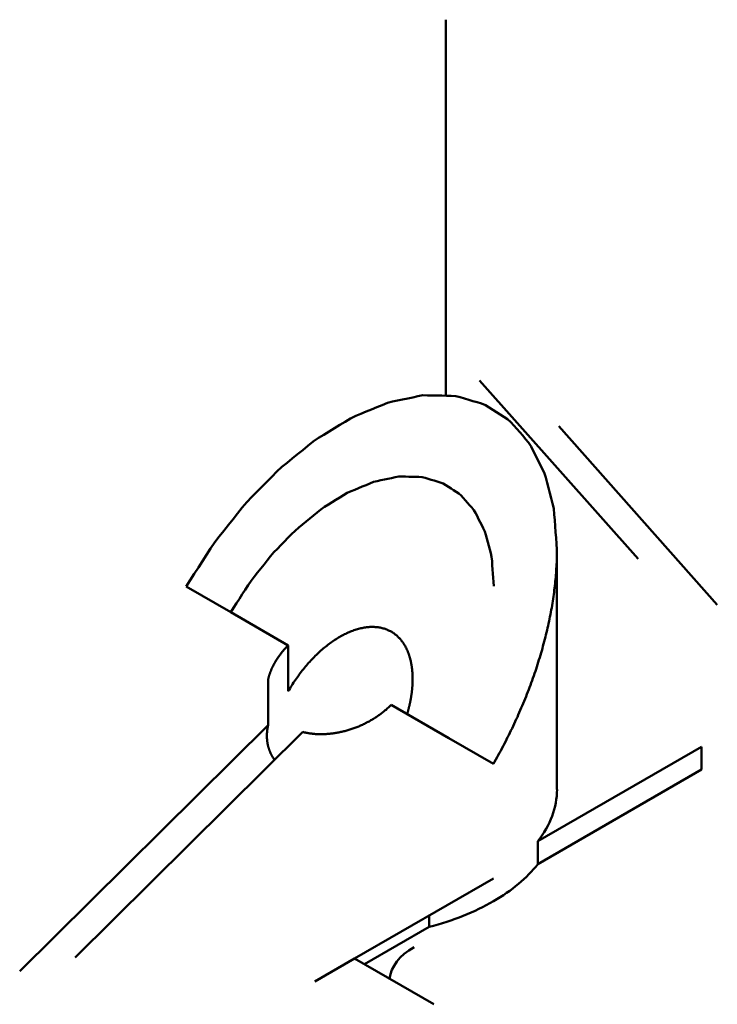
# Model space of a CAD drawing. Units: inches. Extents: x 181 to 9700, y 72 to 10161.
# Tile 2 of 2: x 5829 to 9700, y 4700 to 10161. Entities that reach past the tile are written whole.
import ezdxf

# ---------------------------------------------------------------- set-up
doc = ezdxf.new("R2010")
doc.units = ezdxf.units.IN
doc.header["$MEASUREMENT"] = 0
doc.layers.add('M-OUTL', color=7, linetype='Continuous', lineweight=50)

msp = doc.modelspace()

# ---------------------------------------------------------------- linework, layer by layer
at = {"layer": 'M-OUTL'}
for p, q in [((8193.3, 8080.4), (8193.3, 10161.2)), ((9260.1, 7170.3), (8380.2, 8160.9)), ((9700.1, 6916.3), (8820.2, 7906.9)), ((8810.3, 7221.8), (8810.3, 5890.8)), ((6999.9, 6875), (6752.5, 7017.9)), ((7318.9, 6690.9), (6999.9, 6875)), ((7318.9, 6436.9), (7318.9, 6690.9)), ((7207.6, 6249.2), (7207.6, 6503.2)), ((8209.8, 6176.5), (7890.8, 6360.7)), ((5828.6, 4884.3), (7207.6, 6249.2)), ((7399.5, 6210.5), (6136.6, 4960.5)), ((8457.2, 6033.7), (8209.8, 6176.5)), ((8703.5, 5604.3), (9612.1, 6128.9)), ((9612.1, 6001.9), (9612.1, 6128.9)), ((8703.5, 5477.3), (9612.1, 6001.9)), ((8703.5, 5477.3), (8703.5, 5604.3)), ((8457.2, 5398.7), (7687.3, 4954.2)), ((8101, 5129.5), (8101, 5193)), ((7742.3, 4922.4), (8101, 5129.5)), ((7467.4, 4827.2), (7687.3, 4954.2)), ((8127.3, 4700.2), (7687.3, 4954.2))]:
    msp.add_line(p, q, dxfattribs=at)
for points in [[(6752.5, 7017.9), (6775, 7053), (6797.6, 7088), (6820.2, 7123.1), (6842.8, 7158.1), (6865.4, 7193.2), (6887.9, 7228.2), (6910.9, 7262.8), (6936.4, 7294.9), (6961.8, 7326.9), (6987.3, 7358.9), (7012.7, 7391), (7038.2, 7423), (7063.6, 7455), (7089.7, 7485.9), (7117.3, 7514.1), (7144.9, 7542.2), (7172.5, 7570.3), (7200.1, 7598.4), (7227.8, 7626.5), (7255.4, 7654.6), (7283.6, 7680.7), (7312.5, 7704.1), (7341.5, 7727.5), (7370.5, 7750.9), (7399.5, 7774.3), (7428.5, 7797.6), (7457.5, 7821), (7486.8, 7841.3), (7516.3, 7859.4), (7545.8, 7877.4), (7575.4, 7895.4), (7604.9, 7913.4), (7634.5, 7931.4), (7664, 7949.4), (7693.3, 7963.2), (7722.6, 7975.4), (7751.9, 7987.5), (7781.1, 7999.6), (7810.4, 8011.7), (7839.7, 8023.8), (7868.9, 8036), (7897.2, 8042.8), (7925.4, 8048.6), (7953.5, 8054.5), (7981.7, 8060.4), (8009.8, 8066.3), (8038, 8072.2), (8066.2, 8078.1), (8092.4, 8077.6), (8118.7, 8077.1), (8144.9, 8076.6), (8171.2, 8076.1), (8197.4, 8075.6), (8223.7, 8075.1), (8249.6, 8073.7), (8273.2, 8066.8), (8296.8, 8059.9), (8320.4, 8053), (8344, 8046.1), (8367.6, 8039.2), (8391.2, 8032.4), (8413.9, 8023.7), (8434.2, 8010.6), (8454.5, 7997.6), (8474.8, 7984.5), (8495.1, 7971.4), (8515.4, 7958.3), (8535.7, 7945.3), (8554.4, 7929.7), (8570.8, 7910.8), (8587.2, 7891.9), (8603.6, 7873), (8620, 7854.1), (8636.4, 7835.2), (8652.9, 7816.3), (8666.8, 7794.4), (8678.9, 7770.2), (8690.9, 7746.1), (8703, 7721.9), (8715.1, 7697.7), (8727.1, 7673.5), (8739.2, 7649.3), (8747.9, 7621.9), (8755.3, 7593.1), (8762.7, 7564.3), (8770.1, 7535.5), (8777.5, 7506.8), (8784.8, 7478), (8792.2, 7449.2), (8795.4, 7417.2), (8797.9, 7384.6), (8800.4, 7352), (8802.9, 7319.5), (8805.3, 7286.9), (8807.8, 7254.3), (8810.3, 7221.8)], [(6999.9, 6875), (7016, 6899.9), (7032, 6924.8), (7048, 6949.7), (7064, 6974.5), (7080.1, 6999.4), (7096.1, 7024.3), (7112.4, 7048.9), (7130.5, 7071.6), (7148.5, 7094.3), (7166.6, 7117.1), (7184.6, 7139.8), (7202.7, 7162.5), (7220.8, 7185.3), (7239.3, 7207.2), (7258.9, 7227.1), (7278.5, 7247.1), (7298.1, 7267), (7317.6, 7287), (7337.2, 7306.9), (7356.8, 7326.9), (7376.8, 7345.4), (7397.4, 7362), (7418, 7378.6), (7438.5, 7395.2), (7459.1, 7411.8), (7479.7, 7428.4), (7500.3, 7445), (7521, 7459.4), (7542, 7472.2), (7563, 7485), (7583.9, 7497.8), (7604.9, 7510.5), (7625.9, 7523.3), (7646.8, 7536.1), (7667.7, 7545.9), (7688.4, 7554.5), (7709.2, 7563.1), (7730, 7571.7), (7750.7, 7580.3), (7771.5, 7588.9), (7792.3, 7597.5), (7812.3, 7602.3), (7832.3, 7606.5), (7852.3, 7610.7), (7872.3, 7614.9), (7892.3, 7619.1), (7912.3, 7623.3), (7932.2, 7627.4), (7950.9, 7627.1), (7969.5, 7626.7), (7988.1, 7626.4), (8006.8, 7626), (8025.4, 7625.7), (8044, 7625.3), (8062.4, 7624.3), (8079.1, 7619.4), (8095.9, 7614.5), (8112.7, 7609.6), (8129.4, 7604.7), (8146.2, 7599.9), (8162.9, 7595), (8179, 7588.8), (8193.4, 7579.5), (8207.8, 7570.3), (8222.2, 7561), (8236.6, 7551.7), (8251.1, 7542.4), (8265.5, 7533.2), (8278.7, 7522.1), (8290.3, 7508.7), (8302, 7495.3), (8313.6, 7481.9), (8325.3, 7468.5), (8336.9, 7455.1), (8348.6, 7441.7), (8358.5, 7426.1), (8367.1, 7408.9), (8375.6, 7391.8), (8384.2, 7374.6), (8392.8, 7357.5), (8401.3, 7340.3), (8409.9, 7323.2), (8416.1, 7303.7), (8421.3, 7283.2), (8426.5, 7262.8), (8431.8, 7242.4), (8437, 7222), (8442.3, 7201.5), (8447.5, 7181.1), (8449.8, 7158.4), (8451.5, 7135.3), (8453.3, 7112.2), (8455, 7089), (8456.8, 7065.9), (8458.6, 7042.8), (8460.3, 7019.7)], [(8810.3, 7221.8), (8810, 7210.2), (8809.8, 7198.7), (8809.5, 7187.1), (8809.2, 7175.6), (8808.9, 7164.1), (8808.6, 7152.5), (8808.3, 7140.9), (8807.5, 7129.1), (8806.6, 7117.3), (8805.8, 7105.5), (8805, 7093.6), (8804.1, 7081.8), (8803.3, 7070), (8802.3, 7058.1), (8801, 7046), (8799.6, 7034), (8798.2, 7021.9), (8796.8, 7009.8), (8795.4, 6997.7), (8794.1, 6985.7), (8792.5, 6973.5), (8790.5, 6961.2), (8788.6, 6949), (8786.7, 6936.7), (8784.8, 6924.4), (8782.8, 6912.1), (8780.9, 6899.8), (8778.7, 6887.5), (8776.2, 6875), (8773.8, 6862.6), (8771.3, 6850.1), (8768.8, 6837.7), (8766.4, 6825.2), (8763.9, 6812.8), (8761.1, 6800.2), (8758.1, 6787.7), (8755.1, 6775.1), (8752.1, 6762.5), (8749.1, 6749.9), (8746.1, 6737.4), (8743.1, 6724.8), (8739.6, 6712.1), (8736.1, 6699.5), (8732.6, 6686.8), (8729.1, 6674.1), (8725.6, 6661.4), (8722.1, 6648.8), (8718.5, 6636.1), (8714.5, 6623.4), (8710.5, 6610.7), (8706.5, 6598), (8702.4, 6585.2), (8698.4, 6572.5), (8694.4, 6559.8), (8690.3, 6547.1), (8685.8, 6534.4), (8681.2, 6521.6), (8676.7, 6508.9), (8672.2, 6496.2), (8667.7, 6483.4), (8663.1, 6470.7), (8658.5, 6458), (8653.5, 6445.3), (8648.4, 6432.6), (8643.4, 6419.9), (8638.4, 6407.2), (8633.4, 6394.5), (8628.4, 6381.8), (8623.2, 6369.1), (8617.7, 6356.5), (8612.2, 6343.9), (8606.8, 6331.2), (8601.3, 6318.6), (8595.8, 6306), (8590.3, 6293.3), (8584.6, 6280.8), (8578.7, 6268.2), (8572.7, 6255.7), (8566.8, 6243.2), (8560.9, 6230.7), (8554.9, 6218.2), (8549, 6205.6), (8542.8, 6193.2), (8536.4, 6180.9), (8530, 6168.5), (8523.7, 6156.1), (8517.3, 6143.7), (8511, 6131.4), (8504.6, 6119), (8497.9, 6106.8), (8491.1, 6094.6), (8484.3, 6082.4), (8477.6, 6070.2), (8470.8, 6058), (8464, 6045.9), (8457.2, 6033.7)], [(7318.9, 6436.9), (7323.8, 6444.8), (7328.8, 6452.8), (7333.7, 6460.7), (7338.6, 6468.6), (7343.5, 6476.6), (7348.5, 6484.5), (7353.5, 6492.4), (7358.9, 6499.9), (7364.3, 6507.5), (7369.7, 6515), (7375.1, 6522.5), (7380.4, 6530.1), (7385.8, 6537.6), (7391.3, 6545), (7397.1, 6552), (7402.9, 6559.1), (7408.7, 6566.1), (7414.5, 6573.1), (7420.3, 6580.2), (7426.1, 6587.2), (7432, 6594), (7438.1, 6600.4), (7444.2, 6606.9), (7450.3, 6613.3), (7456.4, 6619.8), (7462.6, 6626.2), (7468.7, 6632.7), (7474.9, 6638.8), (7481.3, 6644.5), (7487.6, 6650.3), (7494, 6656.1), (7500.3, 6661.9), (7506.7, 6667.7), (7513, 6673.5), (7519.5, 6678.7), (7526, 6683.7), (7532.6, 6688.8), (7539.1, 6693.8), (7545.6, 6698.9), (7552.1, 6703.9), (7558.6, 6709), (7565.2, 6713.3), (7571.8, 6717.6), (7578.4, 6721.8), (7585, 6726), (7591.6, 6730.3), (7598.3, 6734.5), (7604.9, 6738.8), (7611.5, 6742.2), (7618.1, 6745.5), (7624.7, 6748.9), (7631.3, 6752.3), (7637.9, 6755.7), (7644.5, 6759.1), (7651.1, 6762.3), (7657.6, 6764.8), (7664.1, 6767.3), (7670.6, 6769.8), (7677.1, 6772.3), (7683.7, 6774.8), (7690.2, 6777.2), (7696.7, 6779.5), (7703, 6781), (7709.4, 6782.6), (7715.7, 6784.1), (7722.1, 6785.7), (7728.4, 6787.2), (7734.8, 6788.8), (7741, 6789.9), (7747.2, 6790.5), (7753.3, 6791.1), (7759.4, 6791.8), (7765.5, 6792.4), (7771.6, 6793), (7777.7, 6793.6), (7783.6, 6793.6), (7789.4, 6793.3), (7795.2, 6792.9), (7801, 6792.6), (7806.8, 6792.2), (7812.6, 6791.9), (7818.4, 6791.5), (7823.9, 6790.5), (7829.3, 6789.2), (7834.7, 6787.9), (7840, 6786.6), (7845.4, 6785.3), (7850.8, 6784), (7856.2, 6782.7), (7861.2, 6780.5), (7866.2, 6778.3), (7871.1, 6776.1), (7876, 6773.8), (7881, 6771.6), (7885.9, 6769.3), (7890.8, 6767.1)], [(7890.8, 6767.1), (7893.1, 6765.6), (7895.4, 6764.2), (7897.6, 6762.7), (7899.9, 6761.2), (7902.2, 6759.8), (7904.5, 6758.3), (7906.7, 6756.8), (7908.8, 6755.1), (7911, 6753.4), (7913.1, 6751.8), (7915.2, 6750.1), (7917.4, 6748.4), (7919.5, 6746.7), (7921.6, 6744.9), (7923.6, 6743), (7925.6, 6741.1), (7927.6, 6739.2), (7929.6, 6737.3), (7931.5, 6735.4), (7933.5, 6733.5), (7935.5, 6731.5), (7937.3, 6729.4), (7939.1, 6727.3), (7941, 6725.2), (7942.8, 6723.1), (7944.7, 6721), (7946.5, 6718.8), (7948.2, 6716.6), (7949.9, 6714.3), (7951.6, 6712), (7953.3, 6709.7), (7955, 6707.3), (7956.6, 6705), (7958.3, 6702.7), (7959.9, 6700.2), (7961.4, 6697.7), (7962.9, 6695.2), (7964.4, 6692.7), (7966, 6690.2), (7967.5, 6687.6), (7969, 6685.1), (7970.4, 6682.4), (7971.7, 6679.7), (7973.1, 6677), (7974.4, 6674.3), (7975.8, 6671.6), (7977.1, 6668.9), (7978.5, 6666.2), (7979.7, 6663.3), (7980.8, 6660.4), (7982, 6657.5), (7983.2, 6654.7), (7984.4, 6651.8), (7985.6, 6648.9), (7986.7, 6646), (7987.7, 6642.9), (7988.7, 6639.9), (7989.7, 6636.8), (7990.7, 6633.7), (7991.7, 6630.7), (7992.7, 6627.6), (7993.7, 6624.5), (7994.5, 6621.3), (7995.3, 6618.1), (7996.2, 6614.8), (7997, 6611.6), (7997.8, 6608.4), (7998.7, 6605.2), (7999.4, 6601.9), (8000, 6598.5), (8000.7, 6595.1), (8001.3, 6591.8), (8002, 6588.4), (8002.6, 6585), (8003.3, 6581.6), (8003.8, 6578.2), (8004.3, 6574.7), (8004.7, 6571.2), (8005.2, 6567.6), (8005.7, 6564.1), (8006.1, 6560.6), (8006.6, 6557.1), (8006.9, 6553.5), (8007.2, 6549.8), (8007.5, 6546.2), (8007.8, 6542.6), (8008, 6538.9), (8008.3, 6535.3), (8008.6, 6531.6), (8008.7, 6527.9), (8008.8, 6524.1), (8008.9, 6520.3), (8009, 6516.6), (8009.1, 6512.8), (8009.2, 6509), (8009.3, 6505.3)], [(7207.6, 6503.2), (7208.1, 6505.2), (7208.6, 6507.2), (7209.2, 6509.3), (7209.7, 6511.3), (7210.2, 6513.3), (7210.7, 6515.4), (7211.3, 6517.4), (7211.9, 6519.5), (7212.5, 6521.5), (7213.1, 6523.5), (7213.8, 6525.6), (7214.4, 6527.6), (7215, 6529.6), (7215.7, 6531.7), (7216.4, 6533.7), (7217.1, 6535.8), (7217.9, 6537.8), (7218.6, 6539.8), (7219.3, 6541.9), (7220.1, 6543.9), (7220.8, 6545.9), (7221.7, 6548), (7222.5, 6550), (7223.3, 6552), (7224.2, 6554.1), (7225, 6556.1), (7225.8, 6558.1), (7226.7, 6560.2), (7227.7, 6562.2), (7228.6, 6564.2), (7229.5, 6566.2), (7230.5, 6568.2), (7231.4, 6570.3), (7232.3, 6572.3), (7233.3, 6574.3), (7234.4, 6576.3), (7235.4, 6578.3), (7236.4, 6580.3), (7237.5, 6582.3), (7238.5, 6584.4), (7239.5, 6586.4), (7240.6, 6588.4), (7241.8, 6590.4), (7242.9, 6592.4), (7244, 6594.3), (7245.2, 6596.3), (7246.3, 6598.3), (7247.4, 6600.3), (7248.6, 6602.3), (7249.9, 6604.3), (7251.1, 6606.3), (7252.3, 6608.2), (7253.5, 6610.2), (7254.8, 6612.2), (7256, 6614.1), (7257.3, 6616.1), (7258.6, 6618), (7260, 6620), (7261.3, 6621.9), (7262.6, 6623.9), (7263.9, 6625.9), (7265.2, 6627.8), (7266.7, 6629.7), (7268.1, 6631.6), (7269.5, 6633.6), (7270.9, 6635.5), (7272.3, 6637.4), (7273.7, 6639.3), (7275.1, 6641.3), (7276.6, 6643.1), (7278.1, 6645), (7279.6, 6646.9), (7281.1, 6648.8), (7282.6, 6650.7), (7284.1, 6652.6), (7285.6, 6654.5), (7287.2, 6656.3), (7288.8, 6658.2), (7290.4, 6660.1), (7292, 6661.9), (7293.5, 6663.8), (7295.1, 6665.6), (7296.8, 6667.5), (7298.4, 6669.3), (7300.1, 6671.1), (7301.7, 6672.9), (7303.4, 6674.8), (7305.1, 6676.6), (7306.7, 6678.4), (7308.4, 6680.2), (7310.2, 6682), (7311.9, 6683.8), (7313.7, 6685.5), (7315.4, 6687.3), (7317.2, 6689.1), (7318.9, 6690.9)], [(8009.3, 6505.3), (8009.2, 6503.4), (8009.2, 6501.5), (8009.2, 6499.5), (8009.2, 6497.6), (8009.1, 6495.7), (8009.1, 6493.8), (8009.1, 6491.9), (8009, 6489.9), (8009, 6488), (8008.9, 6486.1), (8008.8, 6484.1), (8008.8, 6482.2), (8008.7, 6480.3), (8008.6, 6478.3), (8008.5, 6476.4), (8008.4, 6474.4), (8008.3, 6472.4), (8008.1, 6470.5), (8008, 6468.5), (8007.9, 6466.5), (8007.8, 6464.6), (8007.6, 6462.6), (8007.5, 6460.6), (8007.3, 6458.6), (8007.1, 6456.6), (8007, 6454.7), (8006.8, 6452.7), (8006.6, 6450.7), (8006.4, 6448.7), (8006.2, 6446.7), (8006, 6444.7), (8005.8, 6442.7), (8005.6, 6440.7), (8005.4, 6438.7), (8005.2, 6436.6), (8004.9, 6434.6), (8004.7, 6432.6), (8004.4, 6430.6), (8004.2, 6428.5), (8003.9, 6426.5), (8003.6, 6424.5), (8003.4, 6422.5), (8003.1, 6420.4), (8002.8, 6418.4), (8002.5, 6416.3), (8002.2, 6414.3), (8001.9, 6412.3), (8001.6, 6410.2), (8001.2, 6408.2), (8000.9, 6406.1), (8000.6, 6404.1), (8000.2, 6402), (7999.9, 6399.9), (7999.5, 6397.9), (7999.2, 6395.8), (7998.8, 6393.8), (7998.4, 6391.7), (7998, 6389.6), (7997.6, 6387.5), (7997.2, 6385.5), (7996.9, 6383.4), (7996.5, 6381.3), (7996, 6379.2), (7995.6, 6377.2), (7995.2, 6375.1), (7994.7, 6373), (7994.3, 6370.9), (7993.9, 6368.8), (7993.4, 6366.7), (7992.9, 6364.7), (7992.5, 6362.6), (7992, 6360.5), (7991.5, 6358.4), (7991, 6356.3), (7990.6, 6354.2), (7990.1, 6352.1), (7989.6, 6350), (7989, 6347.9), (7988.5, 6345.8), (7988, 6343.7), (7987.5, 6341.6), (7987, 6339.5), (7986.4, 6337.4), (7985.8, 6335.3), (7985.3, 6333.1), (7984.7, 6331), (7984.2, 6328.9), (7983.6, 6326.8), (7983, 6324.7), (7982.4, 6322.6), (7981.8, 6320.5), (7981.2, 6318.4), (7980.6, 6316.2), (7980, 6314.1), (7979.4, 6312), (7978.8, 6309.9)], [(7890.8, 6360.7), (7886.7, 6356.9), (7882.6, 6353.1), (7878.5, 6349.4), (7874.4, 6345.6), (7870.3, 6341.8), (7866.2, 6338.1), (7862, 6334.3), (7857.6, 6330.8), (7853.2, 6327.3), (7848.7, 6323.7), (7844.3, 6320.2), (7839.8, 6316.7), (7835.4, 6313.2), (7830.9, 6309.7), (7826.1, 6306.5), (7821.4, 6303.2), (7816.7, 6300), (7812, 6296.7), (7807.2, 6293.5), (7802.5, 6290.2), (7797.6, 6287.1), (7792.7, 6284.1), (7787.7, 6281.2), (7782.7, 6278.3), (7777.7, 6275.3), (7772.7, 6272.4), (7767.7, 6269.4), (7762.6, 6266.7), (7757.4, 6264.1), (7752.3, 6261.5), (7747.1, 6258.9), (7741.9, 6256.2), (7736.7, 6253.6), (7731.5, 6251), (7726.2, 6248.7), (7720.8, 6246.4), (7715.5, 6244.2), (7710.1, 6241.9), (7704.8, 6239.7), (7699.4, 6237.4), (7694.1, 6235.1), (7688.6, 6233.2), (7683.1, 6231.3), (7677.7, 6229.5), (7672.2, 6227.6), (7666.7, 6225.7), (7661.3, 6223.8), (7655.8, 6222), (7650.3, 6220.5), (7644.7, 6219), (7639.2, 6217.5), (7633.7, 6216), (7628.1, 6214.5), (7622.6, 6213), (7617.1, 6211.6), (7611.5, 6210.5), (7606, 6209.5), (7600.4, 6208.4), (7594.9, 6207.3), (7589.3, 6206.2), (7583.8, 6205.1), (7578.2, 6204.2), (7572.7, 6203.5), (7567.2, 6202.8), (7561.7, 6202.2), (7556.2, 6201.5), (7550.6, 6200.9), (7545.1, 6200.2), (7539.6, 6199.7), (7534.2, 6199.5), (7528.8, 6199.2), (7523.3, 6199), (7517.9, 6198.7), (7512.5, 6198.5), (7507, 6198.2), (7501.7, 6198.2), (7496.4, 6198.4), (7491.1, 6198.6), (7485.7, 6198.8), (7480.4, 6199), (7475.1, 6199.1), (7469.8, 6199.3), (7464.6, 6199.8), (7459.5, 6200.4), (7454.4, 6201), (7449.2, 6201.6), (7444.1, 6202.2), (7439, 6202.8), (7433.9, 6203.4), (7428.9, 6204.4), (7424, 6205.4), (7419.1, 6206.4), (7414.2, 6207.4), (7409.3, 6208.4), (7404.4, 6209.5), (7399.5, 6210.5)], [(7200.4, 6188.4), (7200.4, 6189), (7200.5, 6189.6), (7200.5, 6190.3), (7200.5, 6190.9), (7200.5, 6191.5), (7200.5, 6192.1), (7200.5, 6192.8), (7200.5, 6193.4), (7200.5, 6194), (7200.5, 6194.6), (7200.5, 6195.3), (7200.6, 6195.9), (7200.6, 6196.5), (7200.6, 6197.1), (7200.6, 6197.8), (7200.7, 6198.4), (7200.7, 6199), (7200.7, 6199.6), (7200.7, 6200.3), (7200.8, 6200.9), (7200.8, 6201.5), (7200.8, 6202.1), (7200.9, 6202.8), (7200.9, 6203.4), (7200.9, 6204), (7201, 6204.7), (7201, 6205.3), (7201.1, 6205.9), (7201.1, 6206.5), (7201.2, 6207.2), (7201.2, 6207.8), (7201.2, 6208.4), (7201.3, 6209.1), (7201.3, 6209.7), (7201.4, 6210.3), (7201.5, 6211), (7201.5, 6211.6), (7201.6, 6212.2), (7201.6, 6212.9), (7201.7, 6213.5), (7201.7, 6214.1), (7201.8, 6214.8), (7201.9, 6215.4), (7202, 6216), (7202, 6216.7), (7202.1, 6217.3), (7202.2, 6217.9), (7202.2, 6218.6), (7202.3, 6219.2), (7202.4, 6219.8), (7202.5, 6220.5), (7202.6, 6221.1), (7202.6, 6221.7), (7202.7, 6222.4), (7202.8, 6223), (7202.9, 6223.6), (7203, 6224.3), (7203.1, 6224.9), (7203.2, 6225.5), (7203.2, 6226.2), (7203.3, 6226.8), (7203.4, 6227.4), (7203.5, 6228.1), (7203.6, 6228.7), (7203.7, 6229.4), (7203.8, 6230), (7203.9, 6230.6), (7204, 6231.3), (7204.1, 6231.9), (7204.3, 6232.5), (7204.4, 6233.2), (7204.5, 6233.8), (7204.6, 6234.5), (7204.7, 6235.1), (7204.8, 6235.7), (7204.9, 6236.4), (7205, 6237), (7205.2, 6237.6), (7205.3, 6238.3), (7205.4, 6238.9), (7205.5, 6239.6), (7205.7, 6240.2), (7205.8, 6240.8), (7205.9, 6241.5), (7206.1, 6242.1), (7206.2, 6242.8), (7206.3, 6243.4), (7206.5, 6244), (7206.6, 6244.7), (7206.7, 6245.3), (7206.9, 6246), (7207, 6246.6), (7207.2, 6247.2), (7207.3, 6247.9), (7207.4, 6248.5), (7207.6, 6249.2)], [(7243, 6055.6), (7242.2, 6056.9), (7241.3, 6058.1), (7240.5, 6059.3), (7239.7, 6060.5), (7238.8, 6061.7), (7238, 6062.9), (7237.1, 6064.1), (7236.4, 6065.3), (7235.6, 6066.6), (7234.8, 6067.8), (7234, 6069), (7233.2, 6070.3), (7232.4, 6071.5), (7231.7, 6072.8), (7230.9, 6074), (7230.2, 6075.3), (7229.5, 6076.6), (7228.8, 6077.8), (7228.1, 6079.1), (7227.3, 6080.4), (7226.6, 6081.7), (7226, 6083), (7225.3, 6084.3), (7224.6, 6085.6), (7224, 6086.9), (7223.3, 6088.2), (7222.6, 6089.5), (7222, 6090.8), (7221.4, 6092.1), (7220.8, 6093.4), (7220.2, 6094.8), (7219.6, 6096.1), (7219, 6097.4), (7218.4, 6098.8), (7217.8, 6100.1), (7217.3, 6101.5), (7216.8, 6102.8), (7216.2, 6104.2), (7215.7, 6105.5), (7215.1, 6106.9), (7214.6, 6108.2), (7214.1, 6109.6), (7213.6, 6111), (7213.1, 6112.4), (7212.7, 6113.8), (7212.2, 6115.2), (7211.7, 6116.5), (7211.2, 6117.9), (7210.8, 6119.3), (7210.4, 6120.7), (7210, 6122.1), (7209.6, 6123.6), (7209.2, 6125), (7208.7, 6126.4), (7208.3, 6127.8), (7208, 6129.2), (7207.6, 6130.6), (7207.3, 6132.1), (7206.9, 6133.5), (7206.6, 6134.9), (7206.2, 6136.4), (7205.9, 6137.8), (7205.6, 6139.2), (7205.3, 6140.7), (7205, 6142.1), (7204.7, 6143.6), (7204.4, 6145.1), (7204.1, 6146.5), (7203.9, 6148), (7203.7, 6149.4), (7203.4, 6150.9), (7203.2, 6152.4), (7203, 6153.9), (7202.8, 6155.3), (7202.5, 6156.8), (7202.3, 6158.3), (7202.2, 6159.8), (7202, 6161.3), (7201.9, 6162.7), (7201.7, 6164.2), (7201.5, 6165.7), (7201.4, 6167.2), (7201.3, 6168.7), (7201.2, 6170.2), (7201.1, 6171.7), (7201, 6173.2), (7200.9, 6174.7), (7200.8, 6176.3), (7200.7, 6177.8), (7200.6, 6179.3), (7200.6, 6180.8), (7200.6, 6182.3), (7200.5, 6183.8), (7200.5, 6185.4), (7200.5, 6186.9), (7200.4, 6188.4)]]:
    msp.add_lwpolyline(points, dxfattribs=at)
for centre, major_axis, start_param, end_param in [((7604.9, 5890.8), (1205.5, 0), 5.858958, 6.283185), ((7604.9, 5763.8), (1205.5, 0), 5.497787, 5.858958), ((7604.9, 5763.8), (1205.5, 0), 5.136617, 5.497787), ((8347.3, 4827.2), (-466.6, 0), 5.497788, 6.227515)]:
    msp.add_ellipse(centre, major_axis=major_axis, ratio=0.57735, start_param=start_param, end_param=end_param, dxfattribs=at)

doc.saveas('drawing.dxf')
